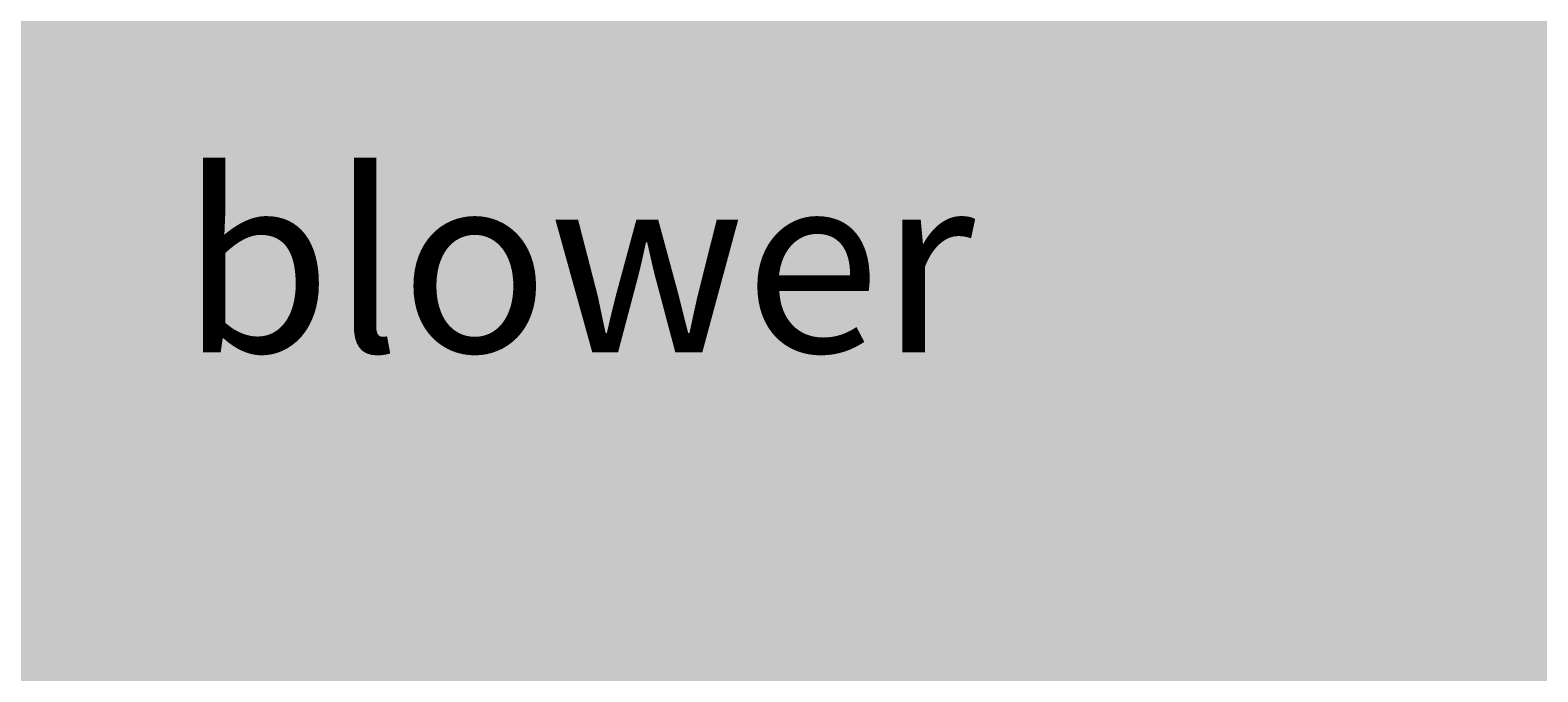
# Model space of a CAD drawing. Units: millimetres. Extents: x -22994 to 29398, y -19990 to 20176.
# Tile 115 of 135: x 220 to 245, y 124 to 135. Entities that reach past the tile are written whole.
import ezdxf

# ---------------------------------------------------------------- set-up
doc = ezdxf.new("R2010")
doc.units = ezdxf.units.MM
doc.header["$MEASUREMENT"] = 0
doc.layers.add('M-ANNO-TEXT', color=7, linetype='Continuous', lineweight=25)
doc.layers.add('M-DIMS', color=2, linetype='Continuous', lineweight=18)
doc.styles.get("Standard").update_dxf_attribs({"font": 'arial.ttf'})
doc.dimstyles.get("Standard").update_dxf_attribs({"dimtxt": 0.18, "dimasz": 10000, "dimexe": 0.18, "dimexo": 0.0625, "dimgap": 0.09, "dimtad": 0, "dimtih": 1, "dimtoh": 1, "dimdec": 0, "dimzin": 0, "dimdsep": 46, "dimtxsty": 'Standard', "dimcen": 0.09, "dimadec": 0, "dimazin": 0, "dimtfac": 1, "dimtdec": 0, "dimtofl": 0, "dimtmove": 0, "dimatfit": 3, "dimfxl": 1, "dimtolj": 1, "dimtzin": 0, "dimlwd": 30, "dimarcsym": 0})

# ---------------------------------------------------------------- blocks, each defined once
blk = doc.blocks.new('*D2')
at = {"layer": 'Defpoints', "color": 0, "transparency": 16777216}
for p in [(6.677, 10.271), (290.852, 10.271), (290.852, -5.079)]:
    blk.add_point(p, dxfattribs=at)
at = {"layer": 'M-DIMS', "color": 0, "lineweight": -2, "transparency": 16777216}
for p, q in [((6.677, 10.209), (6.677, -5.259)), ((290.852, 10.209), (290.852, -5.259))]:
    blk.add_line(p, q, dxfattribs=at)
at = {"layer": 'M-DIMS', "color": 0, "lineweight": 30, "transparency": 16777216}
for p, q in [((-9993.323, -5.079), (-19993.323, -5.079)), ((10290.852, -5.079), (20290.852, -5.079))]:
    blk.add_line(p, q, dxfattribs=at)
at = {"layer": 'M-DIMS', "color": 0, "transparency": 16777216}
for points in [[(-9993.323, 1661.588), (-9993.323, -1671.745), (6.677, -5.079)], [(10290.852, 1661.588), (10290.852, -1671.745), (290.852, -5.079)]]:
    blk.add_solid(points, dxfattribs=at)
at = {"layer": 'M-DIMS', "color": 0, "transparency": 16777216, "insert": (148.765, -5.079), "char_height": 0.18, "attachment_point": 5}
blk.add_mtext('\\A1;284.2', dxfattribs=at)
blk = doc.blocks.new('*D3')
at = {"layer": 'Defpoints', "color": 0, "transparency": 16777216}
for p in [(110.265, 204.165), (110.265, 176.366), (95.833, 127.967)]:
    blk.add_point(p, dxfattribs=at)
at = {"layer": 'M-DIMS', "color": 0, "lineweight": 30, "transparency": 16777216}
for p, q in [((-9904.167, 204.165), (-19904.167, 204.165)), ((10110.265, 204.165), (20110.265, 204.165))]:
    blk.add_line(p, q, dxfattribs=at)
at = {"layer": 'M-DIMS', "color": 0, "lineweight": -2, "transparency": 16777216}
for p, q in [((95.833, 128.03), (95.833, 204.345)), ((110.265, 176.429), (110.265, 204.345))]:
    blk.add_line(p, q, dxfattribs=at)
at = {"layer": 'M-DIMS', "color": 0, "transparency": 16777216}
for points in [[(-9904.167, 1870.832), (-9904.167, -1462.501), (95.833, 204.165)], [(10110.265, 1870.832), (10110.265, -1462.501), (110.265, 204.165)]]:
    blk.add_solid(points, dxfattribs=at)
at = {"layer": 'M-DIMS', "color": 0, "transparency": 16777216, "insert": (103.049, 204.165), "char_height": 0.18, "attachment_point": 5}
blk.add_mtext('\\A1;14.432', dxfattribs=at)
blk = doc.blocks.new('*D4')
at = {"layer": 'Defpoints', "color": 0, "transparency": 16777216}
for p in [(116.265, 204.165), (110.265, 176.366), (116.265, 176.366)]:
    blk.add_point(p, dxfattribs=at)
at = {"layer": 'M-DIMS', "color": 0, "lineweight": 30, "transparency": 16777216}
for p, q in [((-9889.735, 204.165), (-19889.735, 204.165)), ((10116.265, 204.165), (20116.265, 204.165))]:
    blk.add_line(p, q, dxfattribs=at)
at = {"layer": 'M-DIMS', "color": 0, "lineweight": -2, "transparency": 16777216}
for p, q in [((110.265, 176.429), (110.265, 204.345)), ((116.265, 176.429), (116.265, 204.345))]:
    blk.add_line(p, q, dxfattribs=at)
at = {"layer": 'M-DIMS', "color": 0, "transparency": 16777216}
for points in [[(-9889.735, 1870.832), (-9889.735, -1462.501), (110.265, 204.165)], [(10116.265, 1870.832), (10116.265, -1462.501), (116.265, 204.165)]]:
    blk.add_solid(points, dxfattribs=at)
at = {"layer": 'M-DIMS', "color": 0, "transparency": 16777216, "insert": (113.265, 204.165), "char_height": 0.18, "attachment_point": 5}
blk.add_mtext('\\A1;6', dxfattribs=at)
blk = doc.blocks.new('*D5')
at = {"layer": 'Defpoints', "color": 0, "transparency": 16777216}
for p in [(181.265, 204.165), (116.265, 176.366), (181.265, 176.366)]:
    blk.add_point(p, dxfattribs=at)
at = {"layer": 'M-DIMS', "color": 0, "lineweight": 30, "transparency": 16777216}
for p, q in [((-9883.735, 204.165), (-19883.735, 204.165)), ((10181.265, 204.165), (20181.265, 204.165))]:
    blk.add_line(p, q, dxfattribs=at)
at = {"layer": 'M-DIMS', "color": 0, "lineweight": -2, "transparency": 16777216}
for p, q in [((116.265, 176.429), (116.265, 204.345)), ((181.265, 176.429), (181.265, 204.345))]:
    blk.add_line(p, q, dxfattribs=at)
at = {"layer": 'M-DIMS', "color": 0, "transparency": 16777216}
for points in [[(-9883.735, 1870.832), (-9883.735, -1462.501), (116.265, 204.165)], [(10181.265, 1870.832), (10181.265, -1462.501), (181.265, 204.165)]]:
    blk.add_solid(points, dxfattribs=at)
at = {"layer": 'M-DIMS', "color": 0, "transparency": 16777216, "insert": (148.765, 204.165), "char_height": 0.18, "attachment_point": 5}
blk.add_mtext('\\A1;65', dxfattribs=at)
blk = doc.blocks.new('*D6')
at = {"layer": 'Defpoints', "color": 0, "transparency": 16777216}
for p in [(187.265, 204.165), (181.265, 176.366), (187.265, 176.366)]:
    blk.add_point(p, dxfattribs=at)
at = {"layer": 'M-DIMS', "color": 0, "lineweight": 30, "transparency": 16777216}
for p, q in [((-9818.735, 204.165), (-19818.735, 204.165)), ((10187.265, 204.165), (20187.265, 204.165))]:
    blk.add_line(p, q, dxfattribs=at)
at = {"layer": 'M-DIMS', "color": 0, "lineweight": -2, "transparency": 16777216}
for p, q in [((181.265, 176.429), (181.265, 204.345)), ((187.265, 176.429), (187.265, 204.345))]:
    blk.add_line(p, q, dxfattribs=at)
at = {"layer": 'M-DIMS', "color": 0, "transparency": 16777216}
for points in [[(-9818.735, 1870.832), (-9818.735, -1462.501), (181.265, 204.165)], [(10187.265, 1870.832), (10187.265, -1462.501), (187.265, 204.165)]]:
    blk.add_solid(points, dxfattribs=at)
at = {"layer": 'M-DIMS', "color": 0, "transparency": 16777216, "insert": (184.265, 204.165), "char_height": 0.18, "attachment_point": 5}
blk.add_mtext('\\A1;6', dxfattribs=at)
blk = doc.blocks.new('*D7')
at = {"layer": 'Defpoints', "color": 0, "transparency": 16777216}
for p in [(201.697, 204.165), (187.265, 176.366), (201.697, 127.967)]:
    blk.add_point(p, dxfattribs=at)
at = {"layer": 'M-DIMS', "color": 0, "lineweight": 30, "transparency": 16777216}
for p, q in [((-9812.735, 204.165), (-19812.735, 204.165)), ((10201.697, 204.165), (20201.697, 204.165))]:
    blk.add_line(p, q, dxfattribs=at)
at = {"layer": 'M-DIMS', "color": 0, "lineweight": -2, "transparency": 16777216}
for p, q in [((187.265, 176.429), (187.265, 204.345)), ((201.697, 128.03), (201.697, 204.345))]:
    blk.add_line(p, q, dxfattribs=at)
at = {"layer": 'M-DIMS', "color": 0, "transparency": 16777216}
for points in [[(-9812.735, 1870.832), (-9812.735, -1462.501), (187.265, 204.165)], [(10201.697, 1870.832), (10201.697, -1462.501), (201.697, 204.165)]]:
    blk.add_solid(points, dxfattribs=at)
at = {"layer": 'M-DIMS', "color": 0, "transparency": 16777216, "insert": (194.481, 204.165), "char_height": 0.18, "attachment_point": 5}
blk.add_mtext('\\A1;14.432', dxfattribs=at)
blk = doc.blocks.new('*D8')
at = {"layer": 'Defpoints', "color": 0, "transparency": 16777216}
for p in [(227.648, 204.165), (227.648, 146.73), (201.697, 127.967)]:
    blk.add_point(p, dxfattribs=at)
at = {"layer": 'M-DIMS', "color": 0, "lineweight": 30, "transparency": 16777216}
for p, q in [((-9798.303, 204.165), (-19798.303, 204.165)), ((10227.648, 204.165), (20227.648, 204.165))]:
    blk.add_line(p, q, dxfattribs=at)
at = {"layer": 'M-DIMS', "color": 0, "lineweight": -2, "transparency": 16777216}
for p, q in [((201.697, 128.03), (201.697, 204.345)), ((227.648, 146.792), (227.648, 204.345))]:
    blk.add_line(p, q, dxfattribs=at)
at = {"layer": 'M-DIMS', "color": 0, "transparency": 16777216}
for points in [[(-9798.303, 1870.832), (-9798.303, -1462.501), (201.697, 204.165)], [(10227.648, 1870.832), (10227.648, -1462.501), (227.648, 204.165)]]:
    blk.add_solid(points, dxfattribs=at)
at = {"layer": 'M-DIMS', "color": 0, "transparency": 16777216, "insert": (214.673, 204.165), "char_height": 0.18, "attachment_point": 5}
blk.add_mtext('\\A1;25.95', dxfattribs=at)
blk = doc.blocks.new('*D9')
at = {"layer": 'Defpoints', "color": 0, "transparency": 16777216}
for p in [(187.265, 176.366), (306.202, 176.366), (290.852, 10.271)]:
    blk.add_point(p, dxfattribs=at)
at = {"layer": 'M-DIMS', "color": 0, "lineweight": 30, "transparency": 16777216}
for p, q in [((306.202, 10176.366), (306.202, 20176.366)), ((306.202, -9989.729), (306.202, -19989.729))]:
    blk.add_line(p, q, dxfattribs=at)
at = {"layer": 'M-DIMS', "color": 0, "lineweight": -2, "transparency": 16777216}
for p, q in [((187.327, 176.366), (306.382, 176.366)), ((290.915, 10.271), (306.382, 10.271))]:
    blk.add_line(p, q, dxfattribs=at)
at = {"layer": 'M-DIMS', "color": 0, "transparency": 16777216}
for points in [[(-1360.465, 10176.366), (1972.869, 10176.366), (306.202, 176.366)], [(-1360.465, -9989.729), (1972.869, -9989.729), (306.202, 10.271)]]:
    blk.add_solid(points, dxfattribs=at)
at = {"layer": 'M-DIMS', "color": 0, "transparency": 16777216, "insert": (306.202, 93.319), "char_height": 0.18, "attachment_point": 5}
blk.add_mtext('\\A1;166.1', dxfattribs=at)
blk = doc.blocks.new('*D10')
at = {"layer": 'Defpoints', "color": 0, "transparency": 16777216}
for p in [(125.65, 136.071), (133.346, 136.071), (133.346, -5.079)]:
    blk.add_point(p, dxfattribs=at)
at = {"layer": 'M-DIMS', "color": 0, "lineweight": -2, "transparency": 16777216}
for p, q in [((125.65, 136.009), (125.65, -5.259)), ((133.346, 136.009), (133.346, -5.259))]:
    blk.add_line(p, q, dxfattribs=at)
at = {"layer": 'M-DIMS', "color": 0, "lineweight": 30, "transparency": 16777216}
for p, q in [((-9874.35, -5.079), (-19874.35, -5.079)), ((10133.346, -5.079), (20133.346, -5.079))]:
    blk.add_line(p, q, dxfattribs=at)
at = {"layer": 'M-DIMS', "color": 0, "transparency": 16777216}
for points in [[(-9874.35, 1661.588), (-9874.35, -1671.745), (125.65, -5.079)], [(10133.346, 1661.588), (10133.346, -1671.745), (133.346, -5.079)]]:
    blk.add_solid(points, dxfattribs=at)
at = {"layer": 'M-DIMS', "color": 0, "transparency": 16777216, "insert": (129.498, -5.079), "char_height": 0.18, "attachment_point": 5}
blk.add_mtext('\\A1;7.696', dxfattribs=at)
blk = doc.blocks.new('*D11')
at = {"layer": 'Defpoints', "color": 0, "transparency": 16777216}
for p in [(133.346, 136.071), (135.65, 136.071), (135.65, -5.079)]:
    blk.add_point(p, dxfattribs=at)
at = {"layer": 'M-DIMS', "color": 0, "lineweight": -2, "transparency": 16777216}
for p, q in [((133.346, 136.009), (133.346, -5.259)), ((135.65, 136.009), (135.65, -5.259))]:
    blk.add_line(p, q, dxfattribs=at)
at = {"layer": 'M-DIMS', "color": 0, "lineweight": 30, "transparency": 16777216}
for p, q in [((-9866.654, -5.079), (-19866.654, -5.079)), ((10135.65, -5.079), (20135.65, -5.079))]:
    blk.add_line(p, q, dxfattribs=at)
at = {"layer": 'M-DIMS', "color": 0, "transparency": 16777216}
for points in [[(-9866.654, 1661.588), (-9866.654, -1671.745), (133.346, -5.079)], [(10135.65, 1661.588), (10135.65, -1671.745), (135.65, -5.079)]]:
    blk.add_solid(points, dxfattribs=at)
at = {"layer": 'M-DIMS', "color": 0, "transparency": 16777216, "insert": (134.498, -5.079), "char_height": 0.18, "attachment_point": 5}
blk.add_mtext('\\A1;2.304', dxfattribs=at)
blk = doc.blocks.new('*D12')
at = {"layer": 'Defpoints', "color": 0, "transparency": 16777216}
for p in [(135.65, 136.071), (145.65, 136.071), (145.65, -5.079)]:
    blk.add_point(p, dxfattribs=at)
at = {"layer": 'M-DIMS', "color": 0, "lineweight": -2, "transparency": 16777216}
for p, q in [((135.65, 136.009), (135.65, -5.259)), ((145.65, 136.009), (145.65, -5.259))]:
    blk.add_line(p, q, dxfattribs=at)
at = {"layer": 'M-DIMS', "color": 0, "lineweight": 30, "transparency": 16777216}
for p, q in [((-9864.35, -5.079), (-19864.35, -5.079)), ((10145.65, -5.079), (20145.65, -5.079))]:
    blk.add_line(p, q, dxfattribs=at)
at = {"layer": 'M-DIMS', "color": 0, "transparency": 16777216}
for points in [[(-9864.35, 1661.588), (-9864.35, -1671.745), (135.65, -5.079)], [(10145.65, 1661.588), (10145.65, -1671.745), (145.65, -5.079)]]:
    blk.add_solid(points, dxfattribs=at)
at = {"layer": 'M-DIMS', "color": 0, "transparency": 16777216, "insert": (140.65, -5.079), "char_height": 0.18, "attachment_point": 5}
blk.add_mtext('\\A1;10', dxfattribs=at)
blk = doc.blocks.new('*D13')
at = {"layer": 'Defpoints', "color": 0, "transparency": 16777216}
for p in [(145.65, 136.071), (155.65, 136.071), (155.65, -5.079)]:
    blk.add_point(p, dxfattribs=at)
at = {"layer": 'M-DIMS', "color": 0, "lineweight": -2, "transparency": 16777216}
for p, q in [((145.65, 136.009), (145.65, -5.259)), ((155.65, 136.009), (155.65, -5.259))]:
    blk.add_line(p, q, dxfattribs=at)
at = {"layer": 'M-DIMS', "color": 0, "lineweight": 30, "transparency": 16777216}
for p, q in [((-9854.35, -5.079), (-19854.35, -5.079)), ((10155.65, -5.079), (20155.65, -5.079))]:
    blk.add_line(p, q, dxfattribs=at)
at = {"layer": 'M-DIMS', "color": 0, "transparency": 16777216}
for points in [[(-9854.35, 1661.588), (-9854.35, -1671.745), (145.65, -5.079)], [(10155.65, 1661.588), (10155.65, -1671.745), (155.65, -5.079)]]:
    blk.add_solid(points, dxfattribs=at)
at = {"layer": 'M-DIMS', "color": 0, "transparency": 16777216, "insert": (150.65, -5.079), "char_height": 0.18, "attachment_point": 5}
blk.add_mtext('\\A1;10', dxfattribs=at)
blk = doc.blocks.new('*D14')
at = {"layer": 'Defpoints', "color": 0, "transparency": 16777216}
for p in [(155.65, 136.071), (165.65, 136.071), (165.65, -5.079)]:
    blk.add_point(p, dxfattribs=at)
at = {"layer": 'M-DIMS', "color": 0, "lineweight": -2, "transparency": 16777216}
for p, q in [((155.65, 136.009), (155.65, -5.259)), ((165.65, 136.009), (165.65, -5.259))]:
    blk.add_line(p, q, dxfattribs=at)
at = {"layer": 'M-DIMS', "color": 0, "lineweight": 30, "transparency": 16777216}
for p, q in [((-9844.35, -5.079), (-19844.35, -5.079)), ((10165.65, -5.079), (20165.65, -5.079))]:
    blk.add_line(p, q, dxfattribs=at)
at = {"layer": 'M-DIMS', "color": 0, "transparency": 16777216}
for points in [[(-9844.35, 1661.588), (-9844.35, -1671.745), (155.65, -5.079)], [(10165.65, 1661.588), (10165.65, -1671.745), (165.65, -5.079)]]:
    blk.add_solid(points, dxfattribs=at)
at = {"layer": 'M-DIMS', "color": 0, "transparency": 16777216, "insert": (160.65, -5.079), "char_height": 0.18, "attachment_point": 5}
blk.add_mtext('\\A1;10', dxfattribs=at)
blk = doc.blocks.new('*D15')
at = {"layer": 'Defpoints', "color": 0, "transparency": 16777216}
for p in [(173.346, 154.788), (173.346, 136.071), (306.202, 136.071)]:
    blk.add_point(p, dxfattribs=at)
at = {"layer": 'M-DIMS', "color": 0, "lineweight": 30, "transparency": 16777216}
for p, q in [((306.202, 10154.788), (306.202, 20154.788)), ((306.202, -9863.929), (306.202, -19863.929))]:
    blk.add_line(p, q, dxfattribs=at)
at = {"layer": 'M-DIMS', "color": 0, "lineweight": -2, "transparency": 16777216}
for p, q in [((173.408, 154.788), (306.382, 154.788)), ((173.408, 136.071), (306.382, 136.071))]:
    blk.add_line(p, q, dxfattribs=at)
at = {"layer": 'M-DIMS', "color": 0, "transparency": 16777216}
for points in [[(-1360.465, 10154.788), (1972.869, 10154.788), (306.202, 154.788)], [(-1360.465, -9863.929), (1972.869, -9863.929), (306.202, 136.071)]]:
    blk.add_solid(points, dxfattribs=at)
at = {"layer": 'M-DIMS', "color": 0, "transparency": 16777216, "insert": (306.202, 145.43), "char_height": 0.18, "attachment_point": 5}
blk.add_mtext('\\A1;18.717', dxfattribs=at)
blk = doc.blocks.new('*D16')
at = {"layer": 'Defpoints', "color": 0, "transparency": 16777216}
for p in [(120.17, 204.165), (110.466, 48.035), (120.17, 48.035)]:
    blk.add_point(p, dxfattribs=at)
at = {"layer": 'M-DIMS', "color": 0, "lineweight": 30, "transparency": 16777216}
for p, q in [((-9889.534, 204.165), (-19889.534, 204.165)), ((10120.17, 204.165), (20120.17, 204.165))]:
    blk.add_line(p, q, dxfattribs=at)
at = {"layer": 'M-DIMS', "color": 0, "lineweight": -2, "transparency": 16777216}
for p, q in [((110.466, 48.097), (110.466, 204.345)), ((120.17, 48.097), (120.17, 204.345))]:
    blk.add_line(p, q, dxfattribs=at)
at = {"layer": 'M-DIMS', "color": 0, "transparency": 16777216}
for points in [[(-9889.534, 1870.832), (-9889.534, -1462.501), (110.466, 204.165)], [(10120.17, 1870.832), (10120.17, -1462.501), (120.17, 204.165)]]:
    blk.add_solid(points, dxfattribs=at)
at = {"layer": 'M-DIMS', "color": 0, "transparency": 16777216, "insert": (115.318, 204.165), "char_height": 0.18, "attachment_point": 5}
blk.add_mtext('\\A1;9.704', dxfattribs=at)
blk = doc.blocks.new('*D17')
at = {"layer": 'Defpoints', "color": 0, "transparency": 16777216}
for p in [(126.17, 204.165), (120.17, 48.035), (126.17, 48.035)]:
    blk.add_point(p, dxfattribs=at)
at = {"layer": 'M-DIMS', "color": 0, "lineweight": 30, "transparency": 16777216}
for p, q in [((-9879.83, 204.165), (-19879.83, 204.165)), ((10126.17, 204.165), (20126.17, 204.165))]:
    blk.add_line(p, q, dxfattribs=at)
at = {"layer": 'M-DIMS', "color": 0, "lineweight": -2, "transparency": 16777216}
for p, q in [((120.17, 48.097), (120.17, 204.345)), ((126.17, 48.097), (126.17, 204.345))]:
    blk.add_line(p, q, dxfattribs=at)
at = {"layer": 'M-DIMS', "color": 0, "transparency": 16777216}
for points in [[(-9879.83, 1870.832), (-9879.83, -1462.501), (120.17, 204.165)], [(10126.17, 1870.832), (10126.17, -1462.501), (126.17, 204.165)]]:
    blk.add_solid(points, dxfattribs=at)
at = {"layer": 'M-DIMS', "color": 0, "transparency": 16777216, "insert": (123.17, 204.165), "char_height": 0.18, "attachment_point": 5}
blk.add_mtext('\\A1;6', dxfattribs=at)
blk = doc.blocks.new('*D18')
at = {"layer": 'Defpoints', "color": 0, "transparency": 16777216}
for p in [(132.17, 204.165), (126.17, 48.035), (132.17, 48.035)]:
    blk.add_point(p, dxfattribs=at)
at = {"layer": 'M-DIMS', "color": 0, "lineweight": 30, "transparency": 16777216}
for p, q in [((-9873.83, 204.165), (-19873.83, 204.165)), ((10132.17, 204.165), (20132.17, 204.165))]:
    blk.add_line(p, q, dxfattribs=at)
at = {"layer": 'M-DIMS', "color": 0, "lineweight": -2, "transparency": 16777216}
for p, q in [((126.17, 48.097), (126.17, 204.345)), ((132.17, 48.097), (132.17, 204.345))]:
    blk.add_line(p, q, dxfattribs=at)
at = {"layer": 'M-DIMS', "color": 0, "transparency": 16777216}
for points in [[(-9873.83, 1870.832), (-9873.83, -1462.501), (126.17, 204.165)], [(10132.17, 1870.832), (10132.17, -1462.501), (132.17, 204.165)]]:
    blk.add_solid(points, dxfattribs=at)
at = {"layer": 'M-DIMS', "color": 0, "transparency": 16777216, "insert": (129.17, 204.165), "char_height": 0.18, "attachment_point": 5}
blk.add_mtext('\\A1;6', dxfattribs=at)
blk = doc.blocks.new('*D19')
at = {"layer": 'Defpoints', "color": 0, "transparency": 16777216}
for p in [(138.17, 204.165), (132.17, 48.035), (138.17, 48.035)]:
    blk.add_point(p, dxfattribs=at)
at = {"layer": 'M-DIMS', "color": 0, "lineweight": 30, "transparency": 16777216}
for p, q in [((-9867.83, 204.165), (-19867.83, 204.165)), ((10138.17, 204.165), (20138.17, 204.165))]:
    blk.add_line(p, q, dxfattribs=at)
at = {"layer": 'M-DIMS', "color": 0, "lineweight": -2, "transparency": 16777216}
for p, q in [((132.17, 48.097), (132.17, 204.345)), ((138.17, 48.097), (138.17, 204.345))]:
    blk.add_line(p, q, dxfattribs=at)
at = {"layer": 'M-DIMS', "color": 0, "transparency": 16777216}
for points in [[(-9867.83, 1870.832), (-9867.83, -1462.501), (132.17, 204.165)], [(10138.17, 1870.832), (10138.17, -1462.501), (138.17, 204.165)]]:
    blk.add_solid(points, dxfattribs=at)
at = {"layer": 'M-DIMS', "color": 0, "transparency": 16777216, "insert": (135.17, 204.165), "char_height": 0.18, "attachment_point": 5}
blk.add_mtext('\\A1;6', dxfattribs=at)
blk = doc.blocks.new('*D20')
at = {"layer": 'Defpoints', "color": 0, "transparency": 16777216}
for p in [(144.17, 204.165), (138.17, 48.035), (144.17, 48.035)]:
    blk.add_point(p, dxfattribs=at)
at = {"layer": 'M-DIMS', "color": 0, "lineweight": 30, "transparency": 16777216}
for p, q in [((-9861.83, 204.165), (-19861.83, 204.165)), ((10144.17, 204.165), (20144.17, 204.165))]:
    blk.add_line(p, q, dxfattribs=at)
at = {"layer": 'M-DIMS', "color": 0, "lineweight": -2, "transparency": 16777216}
for p, q in [((138.17, 48.097), (138.17, 204.345)), ((144.17, 48.097), (144.17, 204.345))]:
    blk.add_line(p, q, dxfattribs=at)
at = {"layer": 'M-DIMS', "color": 0, "transparency": 16777216}
for points in [[(-9861.83, 1870.832), (-9861.83, -1462.501), (138.17, 204.165)], [(10144.17, 1870.832), (10144.17, -1462.501), (144.17, 204.165)]]:
    blk.add_solid(points, dxfattribs=at)
at = {"layer": 'M-DIMS', "color": 0, "transparency": 16777216, "insert": (141.17, 204.165), "char_height": 0.18, "attachment_point": 5}
blk.add_mtext('\\A1;6', dxfattribs=at)
blk = doc.blocks.new('*D21')
at = {"layer": 'Defpoints', "color": 0, "transparency": 16777216}
for p in [(149.116, 204.165), (144.17, 48.035), (149.116, 48.035)]:
    blk.add_point(p, dxfattribs=at)
at = {"layer": 'M-DIMS', "color": 0, "lineweight": 30, "transparency": 16777216}
for p, q in [((-9855.83, 204.165), (-19855.83, 204.165)), ((10149.116, 204.165), (20149.116, 204.165))]:
    blk.add_line(p, q, dxfattribs=at)
at = {"layer": 'M-DIMS', "color": 0, "lineweight": -2, "transparency": 16777216}
for p, q in [((144.17, 48.097), (144.17, 204.345)), ((149.116, 48.097), (149.116, 204.345))]:
    blk.add_line(p, q, dxfattribs=at)
at = {"layer": 'M-DIMS', "color": 0, "transparency": 16777216}
for points in [[(-9855.83, 1870.832), (-9855.83, -1462.501), (144.17, 204.165)], [(10149.116, 1870.832), (10149.116, -1462.501), (149.116, 204.165)]]:
    blk.add_solid(points, dxfattribs=at)
at = {"layer": 'M-DIMS', "color": 0, "transparency": 16777216, "insert": (146.643, 204.165), "char_height": 0.18, "attachment_point": 5}
blk.add_mtext('\\A1;4.945', dxfattribs=at)
blk = doc.blocks.new('*D22')
at = {"layer": 'Defpoints', "color": 0, "transparency": 16777216}
for p in [(149.116, 30.99), (155.116, 30.99), (155.116, -5.079)]:
    blk.add_point(p, dxfattribs=at)
at = {"layer": 'M-DIMS', "color": 0, "lineweight": -2, "transparency": 16777216}
for p, q in [((149.116, 30.927), (149.116, -5.259)), ((155.116, 30.927), (155.116, -5.259))]:
    blk.add_line(p, q, dxfattribs=at)
at = {"layer": 'M-DIMS', "color": 0, "lineweight": 30, "transparency": 16777216}
for p, q in [((-9850.884, -5.079), (-19850.884, -5.079)), ((10155.116, -5.079), (20155.116, -5.079))]:
    blk.add_line(p, q, dxfattribs=at)
at = {"layer": 'M-DIMS', "color": 0, "transparency": 16777216}
for points in [[(-9850.884, 1661.588), (-9850.884, -1671.745), (149.116, -5.079)], [(10155.116, 1661.588), (10155.116, -1671.745), (155.116, -5.079)]]:
    blk.add_solid(points, dxfattribs=at)
at = {"layer": 'M-DIMS', "color": 0, "transparency": 16777216, "insert": (152.116, -5.079), "char_height": 0.18, "attachment_point": 5}
blk.add_mtext('\\A1;6', dxfattribs=at)
blk = doc.blocks.new('*D23')
at = {"layer": 'Defpoints', "color": 0, "transparency": 16777216}
for p in [(155.116, 30.99), (161.116, 30.99), (161.116, -5.079)]:
    blk.add_point(p, dxfattribs=at)
at = {"layer": 'M-DIMS', "color": 0, "lineweight": -2, "transparency": 16777216}
for p, q in [((155.116, 30.927), (155.116, -5.259)), ((161.116, 30.927), (161.116, -5.259))]:
    blk.add_line(p, q, dxfattribs=at)
at = {"layer": 'M-DIMS', "color": 0, "lineweight": 30, "transparency": 16777216}
for p, q in [((-9844.884, -5.079), (-19844.884, -5.079)), ((10161.116, -5.079), (20161.116, -5.079))]:
    blk.add_line(p, q, dxfattribs=at)
at = {"layer": 'M-DIMS', "color": 0, "transparency": 16777216}
for points in [[(-9844.884, 1661.588), (-9844.884, -1671.745), (155.116, -5.079)], [(10161.116, 1661.588), (10161.116, -1671.745), (161.116, -5.079)]]:
    blk.add_solid(points, dxfattribs=at)
at = {"layer": 'M-DIMS', "color": 0, "transparency": 16777216, "insert": (158.116, -5.079), "char_height": 0.18, "attachment_point": 5}
blk.add_mtext('\\A1;6', dxfattribs=at)
blk = doc.blocks.new('*D24')
at = {"layer": 'Defpoints', "color": 0, "transparency": 16777216}
for p in [(161.116, 30.99), (166.439, 30.99), (166.439, -5.079)]:
    blk.add_point(p, dxfattribs=at)
at = {"layer": 'M-DIMS', "color": 0, "lineweight": -2, "transparency": 16777216}
for p, q in [((161.116, 30.927), (161.116, -5.259)), ((166.439, 30.927), (166.439, -5.259))]:
    blk.add_line(p, q, dxfattribs=at)
at = {"layer": 'M-DIMS', "color": 0, "lineweight": 30, "transparency": 16777216}
for p, q in [((-9838.884, -5.079), (-19838.884, -5.079)), ((10166.439, -5.079), (20166.439, -5.079))]:
    blk.add_line(p, q, dxfattribs=at)
at = {"layer": 'M-DIMS', "color": 0, "transparency": 16777216}
for points in [[(-9838.884, 1661.588), (-9838.884, -1671.745), (161.116, -5.079)], [(10166.439, 1661.588), (10166.439, -1671.745), (166.439, -5.079)]]:
    blk.add_solid(points, dxfattribs=at)
at = {"layer": 'M-DIMS', "color": 0, "transparency": 16777216, "insert": (163.777, -5.079), "char_height": 0.18, "attachment_point": 5}
blk.add_mtext('\\A1;5.323', dxfattribs=at)
blk = doc.blocks.new('*D25')
at = {"layer": 'Defpoints', "color": 0, "transparency": 16777216}
for p in [(166.439, 30.99), (172.439, 30.99), (172.439, -5.079)]:
    blk.add_point(p, dxfattribs=at)
at = {"layer": 'M-DIMS', "color": 0, "lineweight": -2, "transparency": 16777216}
for p, q in [((166.439, 30.927), (166.439, -5.259)), ((172.439, 30.927), (172.439, -5.259))]:
    blk.add_line(p, q, dxfattribs=at)
at = {"layer": 'M-DIMS', "color": 0, "lineweight": 30, "transparency": 16777216}
for p, q in [((-9833.561, -5.079), (-19833.561, -5.079)), ((10172.439, -5.079), (20172.439, -5.079))]:
    blk.add_line(p, q, dxfattribs=at)
at = {"layer": 'M-DIMS', "color": 0, "transparency": 16777216}
for points in [[(-9833.561, 1661.588), (-9833.561, -1671.745), (166.439, -5.079)], [(10172.439, 1661.588), (10172.439, -1671.745), (172.439, -5.079)]]:
    blk.add_solid(points, dxfattribs=at)
at = {"layer": 'M-DIMS', "color": 0, "transparency": 16777216, "insert": (169.439, -5.079), "char_height": 0.18, "attachment_point": 5}
blk.add_mtext('\\A1;6', dxfattribs=at)
blk = doc.blocks.new('*D26')
at = {"layer": 'Defpoints', "color": 0, "transparency": 16777216}
for p in [(172.439, 30.99), (178.439, 30.99), (178.439, -5.079)]:
    blk.add_point(p, dxfattribs=at)
at = {"layer": 'M-DIMS', "color": 0, "lineweight": -2, "transparency": 16777216}
for p, q in [((172.439, 30.927), (172.439, -5.259)), ((178.439, 30.927), (178.439, -5.259))]:
    blk.add_line(p, q, dxfattribs=at)
at = {"layer": 'M-DIMS', "color": 0, "lineweight": 30, "transparency": 16777216}
for p, q in [((-9827.561, -5.079), (-19827.561, -5.079)), ((10178.439, -5.079), (20178.439, -5.079))]:
    blk.add_line(p, q, dxfattribs=at)
at = {"layer": 'M-DIMS', "color": 0, "transparency": 16777216}
for points in [[(-9827.561, 1661.588), (-9827.561, -1671.745), (172.439, -5.079)], [(10178.439, 1661.588), (10178.439, -1671.745), (178.439, -5.079)]]:
    blk.add_solid(points, dxfattribs=at)
at = {"layer": 'M-DIMS', "color": 0, "transparency": 16777216, "insert": (175.439, -5.079), "char_height": 0.18, "attachment_point": 5}
blk.add_mtext('\\A1;6', dxfattribs=at)
blk = doc.blocks.new('*D27')
at = {"layer": 'Defpoints', "color": 0, "transparency": 16777216}
for p in [(178.439, 30.99), (188.117, 30.99), (188.117, -5.079)]:
    blk.add_point(p, dxfattribs=at)
at = {"layer": 'M-DIMS', "color": 0, "lineweight": -2, "transparency": 16777216}
for p, q in [((178.439, 30.927), (178.439, -5.259)), ((188.117, 30.927), (188.117, -5.259))]:
    blk.add_line(p, q, dxfattribs=at)
at = {"layer": 'M-DIMS', "color": 0, "lineweight": 30, "transparency": 16777216}
for p, q in [((-9821.561, -5.079), (-19821.561, -5.079)), ((10188.117, -5.079), (20188.117, -5.079))]:
    blk.add_line(p, q, dxfattribs=at)
at = {"layer": 'M-DIMS', "color": 0, "transparency": 16777216}
for points in [[(-9821.561, 1661.588), (-9821.561, -1671.745), (178.439, -5.079)], [(10188.117, 1661.588), (10188.117, -1671.745), (188.117, -5.079)]]:
    blk.add_solid(points, dxfattribs=at)
at = {"layer": 'M-DIMS', "color": 0, "transparency": 16777216, "insert": (183.278, -5.079), "char_height": 0.18, "attachment_point": 5}
blk.add_mtext('\\A1;9.679', dxfattribs=at)
blk = doc.blocks.new('*D28')
at = {"layer": 'Defpoints', "color": 0, "transparency": 16777216}
for p in [(188.117, 48.035), (306.202, 48.035), (188.117, 30.99)]:
    blk.add_point(p, dxfattribs=at)
at = {"layer": 'M-DIMS', "color": 0, "lineweight": 30, "transparency": 16777216}
for p, q in [((306.202, 10048.035), (306.202, 20048.035)), ((306.202, -9969.01), (306.202, -19969.01))]:
    blk.add_line(p, q, dxfattribs=at)
at = {"layer": 'M-DIMS', "color": 0, "lineweight": -2, "transparency": 16777216}
for p, q in [((188.18, 48.035), (306.382, 48.035)), ((188.18, 30.99), (306.382, 30.99))]:
    blk.add_line(p, q, dxfattribs=at)
at = {"layer": 'M-DIMS', "color": 0, "transparency": 16777216}
for points in [[(-1360.465, 10048.035), (1972.869, 10048.035), (306.202, 48.035)], [(-1360.465, -9969.01), (1972.869, -9969.01), (306.202, 30.99)]]:
    blk.add_solid(points, dxfattribs=at)
at = {"layer": 'M-DIMS', "color": 0, "transparency": 16777216, "insert": (306.202, 39.512), "char_height": 0.18, "attachment_point": 5}
blk.add_mtext('\\A1;17.045', dxfattribs=at)
blk = doc.blocks.new('*D29')
at = {"layer": 'Defpoints', "color": 0, "transparency": 16777216}
for p in [(36.801, 80.045), (64.03, 80.045)]:
    blk.add_point(p, dxfattribs=at)
at = {"layer": 'M-DIMS', "color": 0, "lineweight": -2, "transparency": 16777216}
for p, q in [((50.415, 79.955), (50.415, 80.135)), ((50.325, 80.045), (50.505, 80.045))]:
    blk.add_line(p, q, dxfattribs=at)
at = {"layer": 'M-DIMS', "color": 0, "lineweight": 30, "transparency": 16777216}
blk.add_line((20064.03, 80.03), (10064.03, 80.038), dxfattribs=at)
at = {"layer": 'M-DIMS', "color": 0, "transparency": 16777216}
blk.add_solid([(10064.031, 1746.704), (10064.028, -1586.629), (64.03, 80.045)], dxfattribs=at)
at = {"layer": 'M-DIMS', "color": 0, "transparency": 16777216, "insert": (20064.521, 80.03), "char_height": 0.18, "attachment_point": 5}
blk.add_mtext('\\A1;∅27.23', dxfattribs=at)
blk = doc.blocks.new('*D30')
at = {"layer": 'Defpoints', "color": 0, "transparency": 16777216}
for p in [(216.315, 146.729), (238.982, 146.73)]:
    blk.add_point(p, dxfattribs=at)
at = {"layer": 'M-DIMS', "color": 0, "lineweight": 30, "transparency": 16777216}
blk.add_line((20238.982, 147.496), (10238.982, 147.113), dxfattribs=at)
at = {"layer": 'M-DIMS', "color": 0, "lineweight": -2, "transparency": 16777216}
for p, q in [((227.648, 146.64), (227.648, 146.82)), ((227.558, 146.73), (227.738, 146.73))]:
    blk.add_line(p, q, dxfattribs=at)
at = {"layer": 'M-DIMS', "color": 0, "transparency": 16777216}
blk.add_solid([(10238.918, 1813.78), (10239.046, -1519.554), (238.982, 146.73)], dxfattribs=at)
at = {"layer": 'M-DIMS', "color": 0, "transparency": 16777216, "insert": (20239.544, 147.496), "char_height": 0.18, "attachment_point": 5}
blk.add_mtext('\\A1;∅22.667', dxfattribs=at)
blk = doc.blocks.new('*D31')
at = {"layer": 'Defpoints', "color": 0, "transparency": 16777216}
for p in [(223.164, 146.729), (232.133, 146.73)]:
    blk.add_point(p, dxfattribs=at)
at = {"layer": 'M-DIMS', "color": 0, "lineweight": 30, "transparency": 16777216}
blk.add_line((20232.133, 148.666), (10232.133, 147.698), dxfattribs=at)
at = {"layer": 'M-DIMS', "color": 0, "lineweight": -2, "transparency": 16777216}
for p, q in [((227.648, 146.64), (227.648, 146.82)), ((227.558, 146.73), (227.738, 146.73))]:
    blk.add_line(p, q, dxfattribs=at)
at = {"layer": 'M-DIMS', "color": 0, "transparency": 16777216}
blk.add_solid([(10231.971, 1814.364), (10232.294, -1518.969), (232.133, 146.73)], dxfattribs=at)
at = {"layer": 'M-DIMS', "color": 0, "transparency": 16777216, "insert": (20232.625, 148.666), "char_height": 0.18, "attachment_point": 5}
blk.add_mtext('\\A1;∅8.969', dxfattribs=at)
blk = doc.blocks.new('*D33')
at = {"layer": 'Defpoints', "color": 0, "transparency": 16777216}
for p in [(229.561, 154.377), (232.997, 153.351)]:
    blk.add_point(p, dxfattribs=at)
at = {"layer": 'M-DIMS', "color": 0, "lineweight": -2, "transparency": 16777216}
for p, q in [((229.471, 154.377), (229.651, 154.377)), ((229.561, 154.287), (229.561, 154.467))]:
    blk.add_line(p, q, dxfattribs=at)
at = {"layer": 'M-DIMS', "color": 0, "lineweight": 30, "transparency": 16777216}
for p, q in [((19396.339, -5570.838), (9814.668, -2708.743)), ((29396.339, -5570.838), (19396.339, -5570.838))]:
    blk.add_line(p, q, dxfattribs=at)
at = {"layer": 'M-DIMS', "color": 0, "transparency": 16777216}
blk.add_solid([(10291.684, -1111.798), (9337.652, -4305.689), (232.997, 153.351)], dxfattribs=at)
at = {"layer": 'M-DIMS', "color": 0, "transparency": 16777216, "insert": (29397.012, -5570.838), "char_height": 0.18, "attachment_point": 5}
blk.add_mtext('\\A1;6X R3.586', dxfattribs=at)
blk = doc.blocks.new('*D34')
at = {"layer": 'Defpoints', "color": 0, "transparency": 16777216}
for p in [(178.58, 122.895), (176.812, 121.128)]:
    blk.add_point(p, dxfattribs=at)
at = {"layer": 'M-DIMS', "color": 0, "lineweight": 30, "transparency": 16777216}
for p, q in [((14322.436, 14263.311), (7250.508, 7193.103)), ((24322.436, 14263.311), (14322.436, 14263.311))]:
    blk.add_line(p, q, dxfattribs=at)
at = {"layer": 'M-DIMS', "color": 0, "lineweight": -2, "transparency": 16777216}
for p, q in [((176.722, 121.128), (176.902, 121.128)), ((176.812, 121.038), (176.812, 121.218))]:
    blk.add_line(p, q, dxfattribs=at)
at = {"layer": 'M-DIMS', "color": 0, "transparency": 16777216}
blk.add_solid([(6072.14, 8371.758), (8428.876, 6014.448), (178.58, 122.895)], dxfattribs=at)
at = {"layer": 'M-DIMS', "color": 0, "transparency": 16777216, "insert": (24322.97, 14263.311), "char_height": 0.18, "attachment_point": 5}
blk.add_mtext('\\A1;6X R2.5', dxfattribs=at)
blk = doc.blocks.new('*D36')
at = {"layer": 'Defpoints', "color": 0, "transparency": 16777216}
for p in [(46.39, 31.303), (46.387, 26.593)]:
    blk.add_point(p, dxfattribs=at)
at = {"layer": 'M-DIMS', "color": 0, "lineweight": 30, "transparency": 16777216}
for p, q in [((57.15, 20031.301), (51.77, 10031.302)), ((10057.15, 20031.301), (57.15, 20031.301))]:
    blk.add_line(p, q, dxfattribs=at)
at = {"layer": 'M-DIMS', "color": 0, "lineweight": -2, "transparency": 16777216}
for p, q in [((46.299, 28.948), (46.479, 28.948)), ((46.389, 28.858), (46.389, 29.038))]:
    blk.add_line(p, q, dxfattribs=at)
at = {"layer": 'M-DIMS', "color": 0, "transparency": 16777216}
blk.add_solid([(-1614.896, 10032.199), (1718.436, 10030.405), (46.39, 31.303)], dxfattribs=at)
at = {"layer": 'M-DIMS', "color": 0, "transparency": 16777216, "insert": (10057.554, 20031.301), "char_height": 0.18, "attachment_point": 5}
blk.add_mtext('\\A1;∅4.71', dxfattribs=at)
blk = doc.blocks.new('*D37')
at = {"layer": 'Defpoints', "color": 0, "transparency": 16777216}
for p in [(54.834, 118.615), (59.494, 118.614)]:
    blk.add_point(p, dxfattribs=at)
at = {"layer": 'M-DIMS', "color": 0, "lineweight": -2, "transparency": 16777216}
for p, q in [((57.074, 118.614), (57.254, 118.614)), ((57.164, 118.524), (57.164, 118.704))]:
    blk.add_line(p, q, dxfattribs=at)
at = {"layer": 'M-DIMS', "color": 0, "lineweight": 30, "transparency": 16777216}
blk.add_line((20059.493, 116.253), (10059.494, 117.434), dxfattribs=at)
at = {"layer": 'M-DIMS', "color": 0, "transparency": 16777216}
blk.add_solid([(10059.69, 1784.1), (10059.297, -1549.233), (59.494, 118.614)], dxfattribs=at)
at = {"layer": 'M-DIMS', "color": 0, "transparency": 16777216, "insert": (20059.985, 116.253), "char_height": 0.18, "attachment_point": 5}
blk.add_mtext('\\A1;∅4.659', dxfattribs=at)

msp = doc.modelspace()

# ---------------------------------------------------------------- texts
at = {"layer": 'M-ANNO-TEXT', "insert": (222.4607, 132.85), "char_height": 3, "attachment_point": 1}
msp.add_mtext_dynamic_manual_height_columns('blower', width=37.883315, gutter_width=1, heights=[0], dxfattribs=at)

# ---------------------------------------------------------------- dimensions: what is measured, and where the dimension line sits
at = {"layer": 'M-DIMS'}
for base, p1, p2, override, picture, middle in [((306.202, 176.3662), (290.852, 10.2713), (187.2647, 176.3662), {"dimdec": 1, "dimlfac": 1, "dimrnd": 0, "dimzin": 0, "dimdsep": 46, "dimlunit": 2}, '*D9', (306.202, 93.3187)), ((306.202, 136.0713), (173.3459, 154.788), (173.3459, 136.0713), {"dimdec": 3, "dimlfac": 1, "dimrnd": 0, "dimzin": 0, "dimdsep": 46, "dimlunit": 2}, '*D15', (306.202, 145.4297)), ((306.202, 48.0349), (188.1175, 30.9895), (188.1175, 48.0349), {"dimdec": 3, "dimlfac": 1, "dimrnd": 0, "dimzin": 0, "dimdsep": 46, "dimlunit": 2}, '*D28', (306.202, 39.5122))]:
    dim = msp.add_linear_dim(base=base, p1=p1, p2=p2, angle=90, dimstyle='Standard', override=override, dxfattribs=at)
    dim.commit()
    dim.dimension.update_dxf_attribs({"geometry": picture, "text_midpoint": middle})
for p1, p2, override, picture, middle in [((46.3875, 26.5934), (46.39, 31.3035), {"dimdec": 2, "dimlfac": 1, "dimrnd": 0, "dimzin": 0, "dimdsep": 46, "dimlunit": 2}, '*D36', (10057.5542, 20031.3006)), ((223.1641, 146.7291), (232.1328, 146.73), {"dimdec": 3, "dimlfac": 1, "dimrnd": 0, "dimzin": 0, "dimdsep": 46, "dimlunit": 2}, '*D31', (20232.1327, 148.6656)), ((216.3148, 146.7291), (238.9821, 146.73), {"dimdec": 3, "dimlfac": 1, "dimrnd": 0, "dimzin": 0, "dimdsep": 46, "dimlunit": 2}, '*D30', (20238.9821, 147.4959))]:
    dim = msp.add_diameter_dim_2p(p1=p1, p2=p2, dimstyle='Standard', override=override, dxfattribs=at)
    dim.commit()
    dim.dimension.update_dxf_attribs({"geometry": picture, "text_midpoint": middle, "dimtype": 163})
for center, mpoint, override, picture, middle in [((176.8123, 121.1277), (178.5802, 122.8952), {"dimdec": 1, "dimlfac": 1, "dimrnd": 0, "dimzin": 0, "dimdsep": 46, "dimlunit": 2}, '*D34', (24322.9703, 14263.3108)), ((229.5613, 154.3773), (232.9972, 153.3509), {"dimdec": 3, "dimlfac": 1, "dimrnd": 0, "dimzin": 0, "dimdsep": 46, "dimlunit": 2}, '*D33', (29397.0125, -5570.8378))]:
    dim = msp.add_radius_dim(center=center, mpoint=mpoint, text='6X <>', dimstyle='Standard', override=override, dxfattribs=at)
    dim.commit()
    dim.dimension.update_dxf_attribs({"geometry": picture, "text_midpoint": middle})
for base, p1, p2, override, picture, middle in [((110.2647, 204.1654), (95.8327, 127.967), (110.2647, 176.3662), {"dimdec": 3, "dimlfac": 1, "dimrnd": 0, "dimzin": 0, "dimdsep": 46, "dimlunit": 2}, '*D3', (103.0487, 204.1654)), ((116.2647, 204.1654), (110.2647, 176.3662), (116.2647, 176.3662), {"dimdec": 0, "dimlfac": 1, "dimrnd": 0, "dimzin": 0, "dimdsep": 46, "dimlunit": 2}, '*D4', (113.2647, 204.1654)), ((120.1702, 204.1654), (110.4658, 48.0349), (120.1702, 48.0349), {"dimdec": 3, "dimlfac": 1, "dimrnd": 0, "dimzin": 0, "dimdsep": 46, "dimlunit": 2}, '*D16', (115.318, 204.1654)), ((181.2647, 204.1654), (116.2647, 176.3662), (181.2647, 176.3662), {"dimdec": 0, "dimlfac": 1, "dimrnd": 0, "dimzin": 0, "dimdsep": 46, "dimlunit": 2}, '*D5', (148.7647, 204.1654)), ((126.1702, 204.1654), (120.1702, 48.0349), (126.1702, 48.0349), {"dimdec": 0, "dimlfac": 1, "dimrnd": 0, "dimzin": 0, "dimdsep": 46, "dimlunit": 2}, '*D17', (123.1702, 204.1654)), ((132.1702, 204.1654), (126.1702, 48.0349), (132.1702, 48.0349), {"dimdec": 0, "dimlfac": 1, "dimrnd": 0, "dimzin": 0, "dimdsep": 46, "dimlunit": 2}, '*D18', (129.1702, 204.1654)), ((138.1702, 204.1654), (132.1702, 48.0349), (138.1702, 48.0349), {"dimdec": 0, "dimlfac": 1, "dimrnd": 0, "dimzin": 0, "dimdsep": 46, "dimlunit": 2}, '*D19', (135.1702, 204.1654)), ((144.1702, 204.1654), (138.1702, 48.0349), (144.1702, 48.0349), {"dimdec": 0, "dimlfac": 1, "dimrnd": 0, "dimzin": 0, "dimdsep": 46, "dimlunit": 2}, '*D20', (141.1702, 204.1654)), ((149.11567, 204.16539), (144.17023, 48.03494), (149.11567, 48.03494), {"dimdec": 3, "dimlfac": 1, "dimrnd": 0, "dimzin": 0, "dimdsep": 46, "dimlunit": 2}, '*D21', (146.64295, 204.16539)), ((187.2647, 204.1654), (181.2647, 176.3662), (187.2647, 176.3662), {"dimdec": 0, "dimlfac": 1, "dimrnd": 0, "dimzin": 0, "dimdsep": 46, "dimlunit": 2}, '*D6', (184.2647, 204.1654)), ((201.6967, 204.1654), (187.2647, 176.3662), (201.6967, 127.967), {"dimdec": 3, "dimlfac": 1, "dimrnd": 0, "dimzin": 0, "dimdsep": 46, "dimlunit": 2}, '*D7', (194.4807, 204.1654)), ((227.6485, 204.1654), (201.6967, 127.967), (227.6485, 146.7296), {"dimdec": 2, "dimlfac": 1, "dimrnd": 0, "dimzin": 0, "dimdsep": 46, "dimlunit": 2}, '*D8', (214.6726, 204.1654)), ((290.852, -5.0787), (6.6773, 10.2713), (290.852, 10.2713), {"dimdec": 1, "dimlfac": 1, "dimrnd": 0, "dimzin": 0, "dimdsep": 46, "dimlunit": 2}, '*D2', (148.7647, -5.0787)), ((133.3459, -5.0787), (125.6498, 136.0713), (133.3459, 136.0713), {"dimdec": 3, "dimlfac": 1, "dimrnd": 0, "dimzin": 0, "dimdsep": 46, "dimlunit": 2}, '*D10', (129.4978, -5.0787)), ((135.6498, -5.0787), (133.3459, 136.0713), (135.6498, 136.0713), {"dimdec": 3, "dimlfac": 1, "dimrnd": 0, "dimzin": 0, "dimdsep": 46, "dimlunit": 2}, '*D11', (134.4978, -5.0787)), ((145.6498, -5.0787), (135.6498, 136.0713), (145.6498, 136.0713), {"dimdec": 0, "dimlfac": 1, "dimrnd": 0, "dimzin": 0, "dimdsep": 46, "dimlunit": 2}, '*D12', (140.6498, -5.0787)), ((155.6498, -5.0787), (145.6498, 136.0713), (155.6498, 136.0713), {"dimdec": 0, "dimlfac": 1, "dimrnd": 0, "dimzin": 0, "dimdsep": 46, "dimlunit": 2}, '*D13', (150.6498, -5.0787)), ((155.1157, -5.0787), (149.1157, 30.9895), (155.1157, 30.9895), {"dimdec": 0, "dimlfac": 1, "dimrnd": 0, "dimzin": 0, "dimdsep": 46, "dimlunit": 2}, '*D22', (152.1157, -5.0787)), ((161.1157, -5.0787), (155.1157, 30.9895), (161.1157, 30.9895), {"dimdec": 0, "dimlfac": 1, "dimrnd": 0, "dimzin": 0, "dimdsep": 46, "dimlunit": 2}, '*D23', (158.1157, -5.0787)), ((165.6498, -5.0787), (155.6498, 136.0713), (165.6498, 136.0713), {"dimdec": 0, "dimlfac": 1, "dimrnd": 0, "dimzin": 0, "dimdsep": 46, "dimlunit": 2}, '*D14', (160.6498, -5.0787)), ((166.4387, -5.0787), (161.1157, 30.9895), (166.4387, 30.9895), {"dimdec": 3, "dimlfac": 1, "dimrnd": 0, "dimzin": 0, "dimdsep": 46, "dimlunit": 2}, '*D24', (163.7772, -5.0787)), ((172.4387, -5.0787), (166.4387, 30.9895), (172.4387, 30.9895), {"dimdec": 0, "dimlfac": 1, "dimrnd": 0, "dimzin": 0, "dimdsep": 46, "dimlunit": 2}, '*D25', (169.4387, -5.0787)), ((178.4387, -5.0787), (172.4387, 30.9895), (178.4387, 30.9895), {"dimdec": 0, "dimlfac": 1, "dimrnd": 0, "dimzin": 0, "dimdsep": 46, "dimlunit": 2}, '*D26', (175.4387, -5.0787)), ((188.1175, -5.0787), (178.4387, 30.9895), (188.1175, 30.9895), {"dimdec": 3, "dimlfac": 1, "dimrnd": 0, "dimzin": 0, "dimdsep": 46, "dimlunit": 2}, '*D27', (183.2781, -5.0787))]:
    dim = msp.add_linear_dim(base=base, p1=p1, p2=p2, dimstyle='Standard', override=override, dxfattribs=at)
    dim.commit()
    dim.dimension.update_dxf_attribs({"geometry": picture, "text_midpoint": middle})
for p1, p2, override, picture, middle in [((54.8343, 118.6145), (59.4936, 118.614), {"dimdec": 3, "dimlfac": 1, "dimrnd": 0, "dimzin": 0, "dimdsep": 46, "dimlunit": 2}, '*D37', (20059.4934, 116.2531)), ((36.8006, 80.045), (64.0296, 80.045), {"dimdec": 2, "dimlfac": 1, "dimrnd": 0, "dimzin": 0, "dimdsep": 46, "dimlunit": 2}, '*D29', (20064.0296, 80.0303))]:
    dim = msp.add_diameter_dim_2p(p1=p1, p2=p2, dimstyle='Standard', override=override, dxfattribs=at)
    dim.commit()
    dim.dimension.update_dxf_attribs({"geometry": picture, "text_midpoint": middle})

doc.saveas('drawing.dxf')
